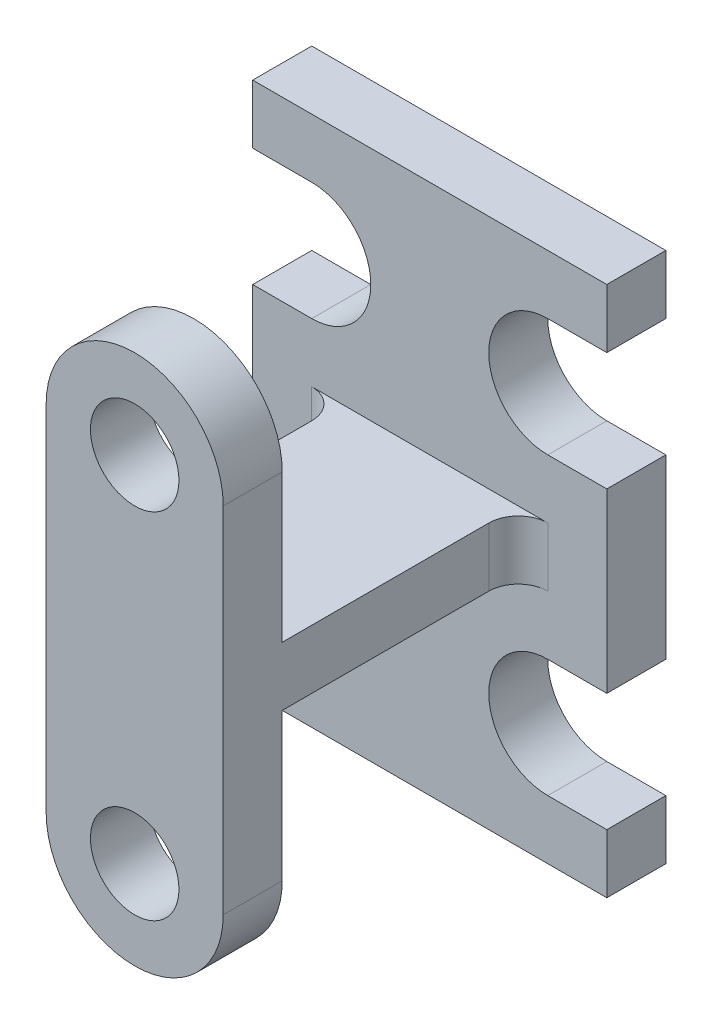
ISO-10303-21;
HEADER;
FILE_DESCRIPTION(('STEP AP214'),'2;1');
FILE_NAME('part.step','',(''),(''),'','','');
FILE_SCHEMA(('AUTOMOTIVE_DESIGN { 1 0 10303 214 1 1 1 1 }'));
ENDSEC;
DATA;
#1=APPLICATION_CONTEXT('core data for automotive mechanical design processes');
#2=APPLICATION_PROTOCOL_DEFINITION('international standard','automotive_design',2000,#1);
#3=PRODUCT_CONTEXT('',#1,'mechanical');
#4=PRODUCT('Part','Part','',(#3));
#5=PRODUCT_RELATED_PRODUCT_CATEGORY('part','',(#4));
#6=PRODUCT_DEFINITION_FORMATION('','',#4);
#7=PRODUCT_DEFINITION_CONTEXT('part definition',#1,'design');
#8=PRODUCT_DEFINITION('design','',#6,#7);
#9=PRODUCT_DEFINITION_SHAPE('','',#8);
#10=(LENGTH_UNIT() NAMED_UNIT(*) SI_UNIT(.MILLI.,.METRE.));
#11=(NAMED_UNIT(*) PLANE_ANGLE_UNIT() SI_UNIT($,.RADIAN.));
#12=(NAMED_UNIT(*) SI_UNIT($,.STERADIAN.) SOLID_ANGLE_UNIT());
#13=UNCERTAINTY_MEASURE_WITH_UNIT(LENGTH_MEASURE(1.E-05),#10,'distance_accuracy_value','');
#14=(GEOMETRIC_REPRESENTATION_CONTEXT(3) GLOBAL_UNCERTAINTY_ASSIGNED_CONTEXT((#13)) GLOBAL_UNIT_ASSIGNED_CONTEXT((#10,
#11,#12)) REPRESENTATION_CONTEXT('',''));
#15=CARTESIAN_POINT('',(0.,0.,0.));
#16=DIRECTION('',(0.,0.,1.));
#17=DIRECTION('',(1.,0.,0.));
#18=AXIS2_PLACEMENT_3D('',#15,#16,#17);
#19=CARTESIAN_POINT('',(3.,-3.5,1.));
#20=DIRECTION('',(-1.,0.,0.));
#21=DIRECTION('',(0.,-1.,0.));
#22=AXIS2_PLACEMENT_3D('',#19,#20,#21);
#23=PLANE('',#22);
#24=DIRECTION('',(0.,1.,0.));
#25=VECTOR('',#24,1.);
#26=CARTESIAN_POINT('',(3.,-3.5,0.));
#27=LINE('',#26,#25);
#28=CARTESIAN_POINT('',(3.,-4.5,0.));
#29=VERTEX_POINT('',#28);
#30=CARTESIAN_POINT('',(3.,-3.5,0.));
#31=VERTEX_POINT('',#30);
#32=EDGE_CURVE('E290',#29,#31,#27,.T.);
#33=ORIENTED_EDGE('',*,*,#32,.T.);
#34=DIRECTION('',(0.,0.,-1.));
#35=VECTOR('',#34,1.);
#36=CARTESIAN_POINT('',(3.,-3.5,1.));
#37=LINE('',#36,#35);
#38=CARTESIAN_POINT('',(3.,-3.5,1.));
#39=VERTEX_POINT('',#38);
#40=EDGE_CURVE('E426',#39,#31,#37,.T.);
#41=ORIENTED_EDGE('',*,*,#40,.F.);
#42=DIRECTION('',(0.,1.,0.));
#43=VECTOR('',#42,1.);
#44=CARTESIAN_POINT('',(3.,-3.5,1.));
#45=LINE('',#44,#43);
#46=CARTESIAN_POINT('',(3.,-4.5,1.));
#47=VERTEX_POINT('',#46);
#48=EDGE_CURVE('E288',#47,#39,#45,.T.);
#49=ORIENTED_EDGE('',*,*,#48,.F.);
#50=DIRECTION('',(0.,0.,-1.));
#51=VECTOR('',#50,1.);
#52=CARTESIAN_POINT('',(3.,-4.5,1.));
#53=LINE('',#52,#51);
#54=EDGE_CURVE('E329',#47,#29,#53,.T.);
#55=ORIENTED_EDGE('',*,*,#54,.T.);
#56=EDGE_LOOP('',(#33,#41,#49,#55));
#57=FACE_BOUND('',#56,.T.);
#58=ADVANCED_FACE('F39',(#57),#23,.F.);
#59=CARTESIAN_POINT('',(2.,-3.5,1.));
#60=DIRECTION('',(0.,-1.,0.));
#61=DIRECTION('',(0.,0.,-1.));
#62=AXIS2_PLACEMENT_3D('',#59,#60,#61);
#63=PLANE('',#62);
#64=DIRECTION('',(-1.,0.,0.));
#65=VECTOR('',#64,1.);
#66=CARTESIAN_POINT('',(2.,-3.5,0.));
#67=LINE('',#66,#65);
#68=CARTESIAN_POINT('',(2.,-3.5,0.));
#69=VERTEX_POINT('',#68);
#70=EDGE_CURVE('E334',#31,#69,#67,.T.);
#71=ORIENTED_EDGE('',*,*,#70,.T.);
#72=DIRECTION('',(0.,0.,-1.));
#73=VECTOR('',#72,1.);
#74=CARTESIAN_POINT('',(2.,-3.5,1.));
#75=LINE('',#74,#73);
#76=CARTESIAN_POINT('',(2.,-3.5,1.));
#77=VERTEX_POINT('',#76);
#78=EDGE_CURVE('E421',#77,#69,#75,.T.);
#79=ORIENTED_EDGE('',*,*,#78,.F.);
#80=DIRECTION('',(-1.,0.,0.));
#81=VECTOR('',#80,1.);
#82=CARTESIAN_POINT('',(2.,-3.5,1.));
#83=LINE('',#82,#81);
#84=EDGE_CURVE('E292',#39,#77,#83,.T.);
#85=ORIENTED_EDGE('',*,*,#84,.F.);
#86=ORIENTED_EDGE('',*,*,#40,.T.);
#87=EDGE_LOOP('',(#71,#79,#85,#86));
#88=FACE_BOUND('',#87,.T.);
#89=ADVANCED_FACE('F499',(#88),#63,.F.);
#90=CARTESIAN_POINT('',(2.,-2.5,1.));
#91=DIRECTION('',(0.,0.,-1.));
#92=DIRECTION('',(-1.,0.,0.));
#93=AXIS2_PLACEMENT_3D('',#90,#91,#92);
#94=CYLINDRICAL_SURFACE('',#93,0.999999999999999);
#95=CARTESIAN_POINT('',(2.,-2.5,0.));
#96=DIRECTION('',(0.,0.,-1.));
#97=DIRECTION('',(1.,0.,0.));
#98=AXIS2_PLACEMENT_3D('',#95,#96,#97);
#99=CIRCLE('',#98,0.999999999999999);
#100=CARTESIAN_POINT('',(2.,-1.5,0.));
#101=VERTEX_POINT('',#100);
#102=EDGE_CURVE('E333',#69,#101,#99,.T.);
#103=ORIENTED_EDGE('',*,*,#102,.T.);
#104=DIRECTION('',(0.,0.,-1.));
#105=VECTOR('',#104,1.);
#106=CARTESIAN_POINT('',(2.,-1.5,1.));
#107=LINE('',#106,#105);
#108=CARTESIAN_POINT('',(2.,-1.5,1.));
#109=VERTEX_POINT('',#108);
#110=EDGE_CURVE('E419',#109,#101,#107,.T.);
#111=ORIENTED_EDGE('',*,*,#110,.F.);
#112=CARTESIAN_POINT('',(2.,-2.5,1.));
#113=DIRECTION('',(0.,0.,-1.));
#114=DIRECTION('',(1.,0.,0.));
#115=AXIS2_PLACEMENT_3D('',#112,#113,#114);
#116=CIRCLE('',#115,0.999999999999999);
#117=EDGE_CURVE('E294',#77,#109,#116,.T.);
#118=ORIENTED_EDGE('',*,*,#117,.F.);
#119=ORIENTED_EDGE('',*,*,#78,.T.);
#120=EDGE_LOOP('',(#103,#111,#118,#119));
#121=FACE_BOUND('',#120,.T.);
#122=ADVANCED_FACE('F504',(#121),#94,.F.);
#123=CARTESIAN_POINT('',(2.,-1.5,1.));
#124=DIRECTION('',(0.,1.,0.));
#125=DIRECTION('',(-1.,0.,0.));
#126=AXIS2_PLACEMENT_3D('',#123,#124,#125);
#127=PLANE('',#126);
#128=DIRECTION('',(1.,0.,0.));
#129=VECTOR('',#128,1.);
#130=CARTESIAN_POINT('',(2.,-1.5,0.));
#131=LINE('',#130,#129);
#132=CARTESIAN_POINT('',(3.,-1.5,0.));
#133=VERTEX_POINT('',#132);
#134=EDGE_CURVE('E340',#101,#133,#131,.T.);
#135=ORIENTED_EDGE('',*,*,#134,.T.);
#136=DIRECTION('',(0.,0.,-1.));
#137=VECTOR('',#136,1.);
#138=CARTESIAN_POINT('',(3.,-1.5,1.));
#139=LINE('',#138,#137);
#140=CARTESIAN_POINT('',(3.,-1.5,1.));
#141=VERTEX_POINT('',#140);
#142=EDGE_CURVE('E417',#141,#133,#139,.T.);
#143=ORIENTED_EDGE('',*,*,#142,.F.);
#144=DIRECTION('',(1.,0.,0.));
#145=VECTOR('',#144,1.);
#146=CARTESIAN_POINT('',(2.,-1.5,1.));
#147=LINE('',#146,#145);
#148=EDGE_CURVE('E298',#109,#141,#147,.T.);
#149=ORIENTED_EDGE('',*,*,#148,.F.);
#150=ORIENTED_EDGE('',*,*,#110,.T.);
#151=EDGE_LOOP('',(#135,#143,#149,#150));
#152=FACE_BOUND('',#151,.T.);
#153=ADVANCED_FACE('F624',(#152),#127,.F.);
#154=CARTESIAN_POINT('',(3.,1.5,1.));
#155=DIRECTION('',(-1.,0.,0.));
#156=DIRECTION('',(0.,-1.,0.));
#157=AXIS2_PLACEMENT_3D('',#154,#155,#156);
#158=PLANE('',#157);
#159=DIRECTION('',(0.,1.,0.));
#160=VECTOR('',#159,1.);
#161=CARTESIAN_POINT('',(3.,1.5,0.));
#162=LINE('',#161,#160);
#163=CARTESIAN_POINT('',(3.,1.5,0.));
#164=VERTEX_POINT('',#163);
#165=EDGE_CURVE('E339',#133,#164,#162,.T.);
#166=ORIENTED_EDGE('',*,*,#165,.T.);
#167=DIRECTION('',(0.,0.,-1.));
#168=VECTOR('',#167,1.);
#169=CARTESIAN_POINT('',(3.,1.5,1.));
#170=LINE('',#169,#168);
#171=CARTESIAN_POINT('',(3.,1.5,1.));
#172=VERTEX_POINT('',#171);
#173=EDGE_CURVE('E414',#172,#164,#170,.T.);
#174=ORIENTED_EDGE('',*,*,#173,.F.);
#175=DIRECTION('',(0.,1.,0.));
#176=VECTOR('',#175,1.);
#177=CARTESIAN_POINT('',(3.,1.5,1.));
#178=LINE('',#177,#176);
#179=EDGE_CURVE('E296',#141,#172,#178,.T.);
#180=ORIENTED_EDGE('',*,*,#179,.F.);
#181=ORIENTED_EDGE('',*,*,#142,.T.);
#182=EDGE_LOOP('',(#166,#174,#180,#181));
#183=FACE_BOUND('',#182,.T.);
#184=ADVANCED_FACE('F616',(#183),#158,.F.);
#185=CARTESIAN_POINT('',(2.,1.5,1.));
#186=DIRECTION('',(0.,-1.,0.));
#187=DIRECTION('',(0.,0.,-1.));
#188=AXIS2_PLACEMENT_3D('',#185,#186,#187);
#189=PLANE('',#188);
#190=DIRECTION('',(-1.,0.,0.));
#191=VECTOR('',#190,1.);
#192=CARTESIAN_POINT('',(2.,1.5,0.));
#193=LINE('',#192,#191);
#194=CARTESIAN_POINT('',(2.,1.5,0.));
#195=VERTEX_POINT('',#194);
#196=EDGE_CURVE('E342',#164,#195,#193,.T.);
#197=ORIENTED_EDGE('',*,*,#196,.T.);
#198=DIRECTION('',(0.,0.,-1.));
#199=VECTOR('',#198,1.);
#200=CARTESIAN_POINT('',(2.,1.5,1.));
#201=LINE('',#200,#199);
#202=CARTESIAN_POINT('',(2.,1.5,1.));
#203=VERTEX_POINT('',#202);
#204=EDGE_CURVE('E412',#203,#195,#201,.T.);
#205=ORIENTED_EDGE('',*,*,#204,.F.);
#206=DIRECTION('',(-1.,0.,0.));
#207=VECTOR('',#206,1.);
#208=CARTESIAN_POINT('',(2.,1.5,1.));
#209=LINE('',#208,#207);
#210=EDGE_CURVE('E297',#172,#203,#209,.T.);
#211=ORIENTED_EDGE('',*,*,#210,.F.);
#212=ORIENTED_EDGE('',*,*,#173,.T.);
#213=EDGE_LOOP('',(#197,#205,#211,#212));
#214=FACE_BOUND('',#213,.T.);
#215=ADVANCED_FACE('F617',(#214),#189,.F.);
#216=CARTESIAN_POINT('',(2.,2.5,1.));
#217=DIRECTION('',(0.,0.,-1.));
#218=DIRECTION('',(-1.,0.,0.));
#219=AXIS2_PLACEMENT_3D('',#216,#217,#218);
#220=CYLINDRICAL_SURFACE('',#219,0.999999999999999);
#221=CARTESIAN_POINT('',(2.,2.5,0.));
#222=DIRECTION('',(0.,0.,-1.));
#223=DIRECTION('',(1.,0.,0.));
#224=AXIS2_PLACEMENT_3D('',#221,#222,#223);
#225=CIRCLE('',#224,0.999999999999999);
#226=CARTESIAN_POINT('',(2.,3.5,0.));
#227=VERTEX_POINT('',#226);
#228=EDGE_CURVE('E343',#195,#227,#225,.T.);
#229=ORIENTED_EDGE('',*,*,#228,.T.);
#230=DIRECTION('',(0.,0.,-1.));
#231=VECTOR('',#230,1.);
#232=CARTESIAN_POINT('',(2.,3.5,1.));
#233=LINE('',#232,#231);
#234=CARTESIAN_POINT('',(2.,3.5,1.));
#235=VERTEX_POINT('',#234);
#236=EDGE_CURVE('E406',#235,#227,#233,.T.);
#237=ORIENTED_EDGE('',*,*,#236,.F.);
#238=CARTESIAN_POINT('',(2.,2.5,1.));
#239=DIRECTION('',(0.,0.,-1.));
#240=DIRECTION('',(1.,0.,0.));
#241=AXIS2_PLACEMENT_3D('',#238,#239,#240);
#242=CIRCLE('',#241,0.999999999999999);
#243=EDGE_CURVE('E305',#203,#235,#242,.T.);
#244=ORIENTED_EDGE('',*,*,#243,.F.);
#245=ORIENTED_EDGE('',*,*,#204,.T.);
#246=EDGE_LOOP('',(#229,#237,#244,#245));
#247=FACE_BOUND('',#246,.T.);
#248=ADVANCED_FACE('F615',(#247),#220,.F.);
#249=CARTESIAN_POINT('',(2.,3.5,1.));
#250=DIRECTION('',(0.,1.,0.));
#251=DIRECTION('',(0.,0.,1.));
#252=AXIS2_PLACEMENT_3D('',#249,#250,#251);
#253=PLANE('',#252);
#254=DIRECTION('',(1.,0.,0.));
#255=VECTOR('',#254,1.);
#256=CARTESIAN_POINT('',(2.,3.5,0.));
#257=LINE('',#256,#255);
#258=CARTESIAN_POINT('',(3.,3.5,0.));
#259=VERTEX_POINT('',#258);
#260=EDGE_CURVE('E341',#227,#259,#257,.T.);
#261=ORIENTED_EDGE('',*,*,#260,.T.);
#262=DIRECTION('',(0.,0.,-1.));
#263=VECTOR('',#262,1.);
#264=CARTESIAN_POINT('',(3.,3.5,1.));
#265=LINE('',#264,#263);
#266=CARTESIAN_POINT('',(3.,3.5,1.));
#267=VERTEX_POINT('',#266);
#268=EDGE_CURVE('E403',#267,#259,#265,.T.);
#269=ORIENTED_EDGE('',*,*,#268,.F.);
#270=DIRECTION('',(1.,0.,0.));
#271=VECTOR('',#270,1.);
#272=CARTESIAN_POINT('',(2.,3.5,1.));
#273=LINE('',#272,#271);
#274=EDGE_CURVE('E304',#235,#267,#273,.T.);
#275=ORIENTED_EDGE('',*,*,#274,.F.);
#276=ORIENTED_EDGE('',*,*,#236,.T.);
#277=EDGE_LOOP('',(#261,#269,#275,#276));
#278=FACE_BOUND('',#277,.T.);
#279=ADVANCED_FACE('F609',(#278),#253,.F.);
#280=CARTESIAN_POINT('',(3.,4.5,1.));
#281=DIRECTION('',(-1.,0.,0.));
#282=DIRECTION('',(0.,-1.,0.));
#283=AXIS2_PLACEMENT_3D('',#280,#281,#282);
#284=PLANE('',#283);
#285=DIRECTION('',(0.,1.,0.));
#286=VECTOR('',#285,1.);
#287=CARTESIAN_POINT('',(3.,4.5,0.));
#288=LINE('',#287,#286);
#289=CARTESIAN_POINT('',(3.,4.5,0.));
#290=VERTEX_POINT('',#289);
#291=EDGE_CURVE('E350',#259,#290,#288,.T.);
#292=ORIENTED_EDGE('',*,*,#291,.T.);
#293=DIRECTION('',(0.,0.,-1.));
#294=VECTOR('',#293,1.);
#295=CARTESIAN_POINT('',(3.,4.5,1.));
#296=LINE('',#295,#294);
#297=CARTESIAN_POINT('',(3.,4.5,1.));
#298=VERTEX_POINT('',#297);
#299=EDGE_CURVE('E405',#298,#290,#296,.T.);
#300=ORIENTED_EDGE('',*,*,#299,.F.);
#301=DIRECTION('',(0.,1.,0.));
#302=VECTOR('',#301,1.);
#303=CARTESIAN_POINT('',(3.,4.5,1.));
#304=LINE('',#303,#302);
#305=EDGE_CURVE('E308',#267,#298,#304,.T.);
#306=ORIENTED_EDGE('',*,*,#305,.F.);
#307=ORIENTED_EDGE('',*,*,#268,.T.);
#308=EDGE_LOOP('',(#292,#300,#306,#307));
#309=FACE_BOUND('',#308,.T.);
#310=ADVANCED_FACE('F603',(#309),#284,.F.);
#311=CARTESIAN_POINT('',(-3.,4.5,1.));
#312=DIRECTION('',(0.,-1.,0.));
#313=DIRECTION('',(0.,0.,-1.));
#314=AXIS2_PLACEMENT_3D('',#311,#312,#313);
#315=PLANE('',#314);
#316=DIRECTION('',(-1.,0.,0.));
#317=VECTOR('',#316,1.);
#318=CARTESIAN_POINT('',(-3.,4.5,0.));
#319=LINE('',#318,#317);
#320=CARTESIAN_POINT('',(-3.,4.5,0.));
#321=VERTEX_POINT('',#320);
#322=EDGE_CURVE('E349',#290,#321,#319,.T.);
#323=ORIENTED_EDGE('',*,*,#322,.T.);
#324=DIRECTION('',(0.,0.,-1.));
#325=VECTOR('',#324,1.);
#326=CARTESIAN_POINT('',(-3.,4.5,1.));
#327=LINE('',#326,#325);
#328=CARTESIAN_POINT('',(-3.,4.5,1.));
#329=VERTEX_POINT('',#328);
#330=EDGE_CURVE('E399',#329,#321,#327,.T.);
#331=ORIENTED_EDGE('',*,*,#330,.F.);
#332=DIRECTION('',(-1.,0.,0.));
#333=VECTOR('',#332,1.);
#334=CARTESIAN_POINT('',(-3.,4.5,1.));
#335=LINE('',#334,#333);
#336=EDGE_CURVE('E306',#298,#329,#335,.T.);
#337=ORIENTED_EDGE('',*,*,#336,.F.);
#338=ORIENTED_EDGE('',*,*,#299,.T.);
#339=EDGE_LOOP('',(#323,#331,#337,#338));
#340=FACE_BOUND('',#339,.T.);
#341=ADVANCED_FACE('F599',(#340),#315,.F.);
#342=CARTESIAN_POINT('',(-3.,4.5,1.));
#343=DIRECTION('',(1.,0.,0.));
#344=DIRECTION('',(0.,0.,-1.));
#345=AXIS2_PLACEMENT_3D('',#342,#343,#344);
#346=PLANE('',#345);
#347=DIRECTION('',(0.,-1.,0.));
#348=VECTOR('',#347,1.);
#349=CARTESIAN_POINT('',(-3.,4.5,0.));
#350=LINE('',#349,#348);
#351=CARTESIAN_POINT('',(-3.,3.5,0.));
#352=VERTEX_POINT('',#351);
#353=EDGE_CURVE('E353',#321,#352,#350,.T.);
#354=ORIENTED_EDGE('',*,*,#353,.T.);
#355=DIRECTION('',(0.,0.,-1.));
#356=VECTOR('',#355,1.);
#357=CARTESIAN_POINT('',(-3.,3.5,1.));
#358=LINE('',#357,#356);
#359=CARTESIAN_POINT('',(-3.,3.5,1.));
#360=VERTEX_POINT('',#359);
#361=EDGE_CURVE('E397',#360,#352,#358,.T.);
#362=ORIENTED_EDGE('',*,*,#361,.F.);
#363=DIRECTION('',(0.,-1.,0.));
#364=VECTOR('',#363,1.);
#365=CARTESIAN_POINT('',(-3.,4.5,1.));
#366=LINE('',#365,#364);
#367=EDGE_CURVE('E309',#329,#360,#366,.T.);
#368=ORIENTED_EDGE('',*,*,#367,.F.);
#369=ORIENTED_EDGE('',*,*,#330,.T.);
#370=EDGE_LOOP('',(#354,#362,#368,#369));
#371=FACE_BOUND('',#370,.T.);
#372=ADVANCED_FACE('F596',(#371),#346,.F.);
#373=CARTESIAN_POINT('',(-3.,3.5,1.));
#374=DIRECTION('',(0.,1.,0.));
#375=DIRECTION('',(0.,0.,1.));
#376=AXIS2_PLACEMENT_3D('',#373,#374,#375);
#377=PLANE('',#376);
#378=DIRECTION('',(1.,0.,0.));
#379=VECTOR('',#378,1.);
#380=CARTESIAN_POINT('',(-3.,3.5,0.));
#381=LINE('',#380,#379);
#382=CARTESIAN_POINT('',(-2.,3.5,0.));
#383=VERTEX_POINT('',#382);
#384=EDGE_CURVE('E351',#352,#383,#381,.T.);
#385=ORIENTED_EDGE('',*,*,#384,.T.);
#386=DIRECTION('',(0.,0.,-1.));
#387=VECTOR('',#386,1.);
#388=CARTESIAN_POINT('',(-2.,3.5,1.));
#389=LINE('',#388,#387);
#390=CARTESIAN_POINT('',(-2.,3.5,1.));
#391=VERTEX_POINT('',#390);
#392=EDGE_CURVE('E391',#391,#383,#389,.T.);
#393=ORIENTED_EDGE('',*,*,#392,.F.);
#394=DIRECTION('',(1.,0.,0.));
#395=VECTOR('',#394,1.);
#396=CARTESIAN_POINT('',(-3.,3.5,1.));
#397=LINE('',#396,#395);
#398=EDGE_CURVE('E315',#360,#391,#397,.T.);
#399=ORIENTED_EDGE('',*,*,#398,.F.);
#400=ORIENTED_EDGE('',*,*,#361,.T.);
#401=EDGE_LOOP('',(#385,#393,#399,#400));
#402=FACE_BOUND('',#401,.T.);
#403=ADVANCED_FACE('F595',(#402),#377,.F.);
#404=CARTESIAN_POINT('',(-2.,2.5,1.));
#405=DIRECTION('',(0.,0.,-1.));
#406=DIRECTION('',(-1.,0.,0.));
#407=AXIS2_PLACEMENT_3D('',#404,#405,#406);
#408=CYLINDRICAL_SURFACE('',#407,0.999999999999999);
#409=CARTESIAN_POINT('',(-2.,2.5,0.));
#410=DIRECTION('',(0.,0.,-1.));
#411=DIRECTION('',(1.,0.,0.));
#412=AXIS2_PLACEMENT_3D('',#409,#410,#411);
#413=CIRCLE('',#412,0.999999999999999);
#414=CARTESIAN_POINT('',(-2.,1.5,0.));
#415=VERTEX_POINT('',#414);
#416=EDGE_CURVE('E352',#383,#415,#413,.T.);
#417=ORIENTED_EDGE('',*,*,#416,.T.);
#418=DIRECTION('',(0.,0.,-1.));
#419=VECTOR('',#418,1.);
#420=CARTESIAN_POINT('',(-2.,1.5,1.));
#421=LINE('',#420,#419);
#422=CARTESIAN_POINT('',(-2.,1.5,1.));
#423=VERTEX_POINT('',#422);
#424=EDGE_CURVE('E388',#423,#415,#421,.T.);
#425=ORIENTED_EDGE('',*,*,#424,.F.);
#426=CARTESIAN_POINT('',(-2.,2.5,1.));
#427=DIRECTION('',(0.,0.,-1.));
#428=DIRECTION('',(1.,0.,0.));
#429=AXIS2_PLACEMENT_3D('',#426,#427,#428);
#430=CIRCLE('',#429,0.999999999999999);
#431=EDGE_CURVE('E314',#391,#423,#430,.T.);
#432=ORIENTED_EDGE('',*,*,#431,.F.);
#433=ORIENTED_EDGE('',*,*,#392,.T.);
#434=EDGE_LOOP('',(#417,#425,#432,#433));
#435=FACE_BOUND('',#434,.T.);
#436=ADVANCED_FACE('F586',(#435),#408,.F.);
#437=CARTESIAN_POINT('',(-3.,1.5,1.));
#438=DIRECTION('',(0.,-1.,0.));
#439=DIRECTION('',(0.,0.,-1.));
#440=AXIS2_PLACEMENT_3D('',#437,#438,#439);
#441=PLANE('',#440);
#442=DIRECTION('',(-1.,0.,0.));
#443=VECTOR('',#442,1.);
#444=CARTESIAN_POINT('',(-3.,1.5,0.));
#445=LINE('',#444,#443);
#446=CARTESIAN_POINT('',(-3.,1.5,0.));
#447=VERTEX_POINT('',#446);
#448=EDGE_CURVE('E360',#415,#447,#445,.T.);
#449=ORIENTED_EDGE('',*,*,#448,.T.);
#450=DIRECTION('',(0.,0.,-1.));
#451=VECTOR('',#450,1.);
#452=CARTESIAN_POINT('',(-3.,1.5,1.));
#453=LINE('',#452,#451);
#454=CARTESIAN_POINT('',(-3.,1.5,1.));
#455=VERTEX_POINT('',#454);
#456=EDGE_CURVE('E390',#455,#447,#453,.T.);
#457=ORIENTED_EDGE('',*,*,#456,.F.);
#458=DIRECTION('',(-1.,0.,0.));
#459=VECTOR('',#458,1.);
#460=CARTESIAN_POINT('',(-3.,1.5,1.));
#461=LINE('',#460,#459);
#462=EDGE_CURVE('E316',#423,#455,#461,.T.);
#463=ORIENTED_EDGE('',*,*,#462,.F.);
#464=ORIENTED_EDGE('',*,*,#424,.T.);
#465=EDGE_LOOP('',(#449,#457,#463,#464));
#466=FACE_BOUND('',#465,.T.);
#467=ADVANCED_FACE('F585',(#466),#441,.F.);
#468=CARTESIAN_POINT('',(-3.,1.5,1.));
#469=DIRECTION('',(1.,0.,0.));
#470=DIRECTION('',(0.,1.,0.));
#471=AXIS2_PLACEMENT_3D('',#468,#469,#470);
#472=PLANE('',#471);
#473=DIRECTION('',(0.,-1.,0.));
#474=VECTOR('',#473,1.);
#475=CARTESIAN_POINT('',(-3.,1.5,0.));
#476=LINE('',#475,#474);
#477=CARTESIAN_POINT('',(-3.,-1.5,0.));
#478=VERTEX_POINT('',#477);
#479=EDGE_CURVE('E359',#447,#478,#476,.T.);
#480=ORIENTED_EDGE('',*,*,#479,.T.);
#481=DIRECTION('',(0.,0.,-1.));
#482=VECTOR('',#481,1.);
#483=CARTESIAN_POINT('',(-3.,-1.5,1.));
#484=LINE('',#483,#482);
#485=CARTESIAN_POINT('',(-3.,-1.5,1.));
#486=VERTEX_POINT('',#485);
#487=EDGE_CURVE('E383',#486,#478,#484,.T.);
#488=ORIENTED_EDGE('',*,*,#487,.F.);
#489=DIRECTION('',(0.,-1.,0.));
#490=VECTOR('',#489,1.);
#491=CARTESIAN_POINT('',(-3.,1.5,1.));
#492=LINE('',#491,#490);
#493=EDGE_CURVE('E318',#455,#486,#492,.T.);
#494=ORIENTED_EDGE('',*,*,#493,.F.);
#495=ORIENTED_EDGE('',*,*,#456,.T.);
#496=EDGE_LOOP('',(#480,#488,#494,#495));
#497=FACE_BOUND('',#496,.T.);
#498=ADVANCED_FACE('F576',(#497),#472,.F.);
#499=CARTESIAN_POINT('',(-3.,-1.5,1.));
#500=DIRECTION('',(0.,1.,0.));
#501=DIRECTION('',(0.,0.,1.));
#502=AXIS2_PLACEMENT_3D('',#499,#500,#501);
#503=PLANE('',#502);
#504=DIRECTION('',(1.,0.,0.));
#505=VECTOR('',#504,1.);
#506=CARTESIAN_POINT('',(-3.,-1.5,0.));
#507=LINE('',#506,#505);
#508=CARTESIAN_POINT('',(-2.,-1.5,0.));
#509=VERTEX_POINT('',#508);
#510=EDGE_CURVE('E363',#478,#509,#507,.T.);
#511=ORIENTED_EDGE('',*,*,#510,.T.);
#512=DIRECTION('',(0.,0.,-1.));
#513=VECTOR('',#512,1.);
#514=CARTESIAN_POINT('',(-2.,-1.5,1.));
#515=LINE('',#514,#513);
#516=CARTESIAN_POINT('',(-2.,-1.5,1.));
#517=VERTEX_POINT('',#516);
#518=EDGE_CURVE('E381',#517,#509,#515,.T.);
#519=ORIENTED_EDGE('',*,*,#518,.F.);
#520=DIRECTION('',(1.,0.,0.));
#521=VECTOR('',#520,1.);
#522=CARTESIAN_POINT('',(-3.,-1.5,1.));
#523=LINE('',#522,#521);
#524=EDGE_CURVE('E319',#486,#517,#523,.T.);
#525=ORIENTED_EDGE('',*,*,#524,.F.);
#526=ORIENTED_EDGE('',*,*,#487,.T.);
#527=EDGE_LOOP('',(#511,#519,#525,#526));
#528=FACE_BOUND('',#527,.T.);
#529=ADVANCED_FACE('F577',(#528),#503,.F.);
#530=CARTESIAN_POINT('',(-2.,-2.5,1.));
#531=DIRECTION('',(0.,0.,-1.));
#532=DIRECTION('',(-1.,0.,0.));
#533=AXIS2_PLACEMENT_3D('',#530,#531,#532);
#534=CYLINDRICAL_SURFACE('',#533,0.999999999999999);
#535=CARTESIAN_POINT('',(-2.,-2.5,0.));
#536=DIRECTION('',(0.,0.,-1.));
#537=DIRECTION('',(1.,0.,0.));
#538=AXIS2_PLACEMENT_3D('',#535,#536,#537);
#539=CIRCLE('',#538,0.999999999999999);
#540=CARTESIAN_POINT('',(-2.,-3.5,0.));
#541=VERTEX_POINT('',#540);
#542=EDGE_CURVE('E361',#509,#541,#539,.T.);
#543=ORIENTED_EDGE('',*,*,#542,.T.);
#544=DIRECTION('',(0.,0.,-1.));
#545=VECTOR('',#544,1.);
#546=CARTESIAN_POINT('',(-2.,-3.5,1.));
#547=LINE('',#546,#545);
#548=CARTESIAN_POINT('',(-2.,-3.5,1.));
#549=VERTEX_POINT('',#548);
#550=EDGE_CURVE('E378',#549,#541,#547,.T.);
#551=ORIENTED_EDGE('',*,*,#550,.F.);
#552=CARTESIAN_POINT('',(-2.,-2.5,1.));
#553=DIRECTION('',(0.,0.,-1.));
#554=DIRECTION('',(1.,0.,0.));
#555=AXIS2_PLACEMENT_3D('',#552,#553,#554);
#556=CIRCLE('',#555,0.999999999999999);
#557=EDGE_CURVE('E325',#517,#549,#556,.T.);
#558=ORIENTED_EDGE('',*,*,#557,.F.);
#559=ORIENTED_EDGE('',*,*,#518,.T.);
#560=EDGE_LOOP('',(#543,#551,#558,#559));
#561=FACE_BOUND('',#560,.T.);
#562=ADVANCED_FACE('F575',(#561),#534,.F.);
#563=CARTESIAN_POINT('',(-3.,-3.5,1.));
#564=DIRECTION('',(0.,-1.,0.));
#565=DIRECTION('',(0.,0.,-1.));
#566=AXIS2_PLACEMENT_3D('',#563,#564,#565);
#567=PLANE('',#566);
#568=DIRECTION('',(-1.,0.,0.));
#569=VECTOR('',#568,1.);
#570=CARTESIAN_POINT('',(-3.,-3.5,0.));
#571=LINE('',#570,#569);
#572=CARTESIAN_POINT('',(-3.,-3.5,0.));
#573=VERTEX_POINT('',#572);
#574=EDGE_CURVE('E364',#541,#573,#571,.T.);
#575=ORIENTED_EDGE('',*,*,#574,.T.);
#576=DIRECTION('',(0.,0.,-1.));
#577=VECTOR('',#576,1.);
#578=CARTESIAN_POINT('',(-3.,-3.5,1.));
#579=LINE('',#578,#577);
#580=CARTESIAN_POINT('',(-3.,-3.5,1.));
#581=VERTEX_POINT('',#580);
#582=EDGE_CURVE('E374',#581,#573,#579,.T.);
#583=ORIENTED_EDGE('',*,*,#582,.F.);
#584=DIRECTION('',(-1.,0.,0.));
#585=VECTOR('',#584,1.);
#586=CARTESIAN_POINT('',(-3.,-3.5,1.));
#587=LINE('',#586,#585);
#588=EDGE_CURVE('E322',#549,#581,#587,.T.);
#589=ORIENTED_EDGE('',*,*,#588,.F.);
#590=ORIENTED_EDGE('',*,*,#550,.T.);
#591=EDGE_LOOP('',(#575,#583,#589,#590));
#592=FACE_BOUND('',#591,.T.);
#593=ADVANCED_FACE('F566',(#592),#567,.F.);
#594=CARTESIAN_POINT('',(-3.,-3.5,1.));
#595=DIRECTION('',(1.,0.,0.));
#596=DIRECTION('',(0.,1.,0.));
#597=AXIS2_PLACEMENT_3D('',#594,#595,#596);
#598=PLANE('',#597);
#599=DIRECTION('',(0.,-1.,0.));
#600=VECTOR('',#599,1.);
#601=CARTESIAN_POINT('',(-3.,-3.5,0.));
#602=LINE('',#601,#600);
#603=CARTESIAN_POINT('',(-3.,-4.5,0.));
#604=VERTEX_POINT('',#603);
#605=EDGE_CURVE('E370',#573,#604,#602,.T.);
#606=ORIENTED_EDGE('',*,*,#605,.T.);
#607=DIRECTION('',(0.,0.,-1.));
#608=VECTOR('',#607,1.);
#609=CARTESIAN_POINT('',(-3.,-4.5,1.));
#610=LINE('',#609,#608);
#611=CARTESIAN_POINT('',(-3.,-4.5,1.));
#612=VERTEX_POINT('',#611);
#613=EDGE_CURVE('E375',#612,#604,#610,.T.);
#614=ORIENTED_EDGE('',*,*,#613,.F.);
#615=DIRECTION('',(0.,-1.,0.));
#616=VECTOR('',#615,1.);
#617=CARTESIAN_POINT('',(-3.,-3.5,1.));
#618=LINE('',#617,#616);
#619=EDGE_CURVE('E326',#581,#612,#618,.T.);
#620=ORIENTED_EDGE('',*,*,#619,.F.);
#621=ORIENTED_EDGE('',*,*,#582,.T.);
#622=EDGE_LOOP('',(#606,#614,#620,#621));
#623=FACE_BOUND('',#622,.T.);
#624=ADVANCED_FACE('F564',(#623),#598,.F.);
#625=CARTESIAN_POINT('',(-3.,-4.5,1.));
#626=DIRECTION('',(0.,1.,0.));
#627=DIRECTION('',(0.,0.,1.));
#628=AXIS2_PLACEMENT_3D('',#625,#626,#627);
#629=PLANE('',#628);
#630=DIRECTION('',(1.,0.,0.));
#631=VECTOR('',#630,1.);
#632=CARTESIAN_POINT('',(-3.,-4.5,0.));
#633=LINE('',#632,#631);
#634=EDGE_CURVE('E295',#604,#29,#633,.T.);
#635=ORIENTED_EDGE('',*,*,#634,.T.);
#636=ORIENTED_EDGE('',*,*,#54,.F.);
#637=DIRECTION('',(1.,0.,0.));
#638=VECTOR('',#637,1.);
#639=CARTESIAN_POINT('',(-3.,-4.5,1.));
#640=LINE('',#639,#638);
#641=EDGE_CURVE('E327',#612,#47,#640,.T.);
#642=ORIENTED_EDGE('',*,*,#641,.F.);
#643=ORIENTED_EDGE('',*,*,#613,.T.);
#644=EDGE_LOOP('',(#635,#636,#642,#643));
#645=FACE_BOUND('',#644,.T.);
#646=ADVANCED_FACE('F559',(#645),#629,.F.);
#647=CARTESIAN_POINT('',(-2.,-2.5,1.));
#648=DIRECTION('',(0.,0.,1.));
#649=DIRECTION('',(1.,0.,0.));
#650=AXIS2_PLACEMENT_3D('',#647,#648,#649);
#651=PLANE('',#650);
#652=DIRECTION('',(1.,0.,0.));
#653=VECTOR('',#652,1.);
#654=CARTESIAN_POINT('',(1.5,-0.5,1.));
#655=LINE('',#654,#653);
#656=CARTESIAN_POINT('',(-2.,-0.5,1.));
#657=VERTEX_POINT('',#656);
#658=CARTESIAN_POINT('',(2.,-0.5,1.));
#659=VERTEX_POINT('',#658);
#660=EDGE_CURVE('E53',#657,#659,#655,.T.);
#661=ORIENTED_EDGE('',*,*,#660,.F.);
#662=DIRECTION('',(0.,-1.,0.));
#663=VECTOR('',#662,1.);
#664=CARTESIAN_POINT('',(-2.,-2.5,1.));
#665=LINE('',#664,#663);
#666=CARTESIAN_POINT('',(-2.,0.5,1.));
#667=VERTEX_POINT('',#666);
#668=EDGE_CURVE('E442',#657,#667,#665,.F.);
#669=ORIENTED_EDGE('',*,*,#668,.T.);
#670=DIRECTION('',(-1.,0.,0.));
#671=VECTOR('',#670,1.);
#672=CARTESIAN_POINT('',(1.5,0.5,1.));
#673=LINE('',#672,#671);
#674=CARTESIAN_POINT('',(2.,0.5,1.));
#675=VERTEX_POINT('',#674);
#676=EDGE_CURVE('E63',#675,#667,#673,.T.);
#677=ORIENTED_EDGE('',*,*,#676,.F.);
#678=DIRECTION('',(0.,1.,0.));
#679=VECTOR('',#678,1.);
#680=CARTESIAN_POINT('',(2.,-2.5,1.));
#681=LINE('',#680,#679);
#682=EDGE_CURVE('E435',#675,#659,#681,.F.);
#683=ORIENTED_EDGE('',*,*,#682,.T.);
#684=EDGE_LOOP('',(#661,#669,#677,#683));
#685=FACE_BOUND('',#684,.T.);
#686=ORIENTED_EDGE('',*,*,#48,.T.);
#687=ORIENTED_EDGE('',*,*,#84,.T.);
#688=ORIENTED_EDGE('',*,*,#117,.T.);
#689=ORIENTED_EDGE('',*,*,#148,.T.);
#690=ORIENTED_EDGE('',*,*,#179,.T.);
#691=ORIENTED_EDGE('',*,*,#210,.T.);
#692=ORIENTED_EDGE('',*,*,#243,.T.);
#693=ORIENTED_EDGE('',*,*,#274,.T.);
#694=ORIENTED_EDGE('',*,*,#305,.T.);
#695=ORIENTED_EDGE('',*,*,#336,.T.);
#696=ORIENTED_EDGE('',*,*,#367,.T.);
#697=ORIENTED_EDGE('',*,*,#398,.T.);
#698=ORIENTED_EDGE('',*,*,#431,.T.);
#699=ORIENTED_EDGE('',*,*,#462,.T.);
#700=ORIENTED_EDGE('',*,*,#493,.T.);
#701=ORIENTED_EDGE('',*,*,#524,.T.);
#702=ORIENTED_EDGE('',*,*,#557,.T.);
#703=ORIENTED_EDGE('',*,*,#588,.T.);
#704=ORIENTED_EDGE('',*,*,#619,.T.);
#705=ORIENTED_EDGE('',*,*,#641,.T.);
#706=EDGE_LOOP('',(#686,#687,#688,#689,#690,#691,#692,#693,#694,#695,#696,#697,#698,#699,#700,
#701,#702,#703,#704,#705));
#707=FACE_BOUND('',#706,.T.);
#708=ADVANCED_FACE('F449',(#685,#707),#651,.T.);
#709=CARTESIAN_POINT('',(-2.,-2.5,0.));
#710=DIRECTION('',(0.,0.,1.));
#711=DIRECTION('',(1.,0.,0.));
#712=AXIS2_PLACEMENT_3D('',#709,#710,#711);
#713=PLANE('',#712);
#714=ORIENTED_EDGE('',*,*,#32,.F.);
#715=ORIENTED_EDGE('',*,*,#634,.F.);
#716=ORIENTED_EDGE('',*,*,#605,.F.);
#717=ORIENTED_EDGE('',*,*,#574,.F.);
#718=ORIENTED_EDGE('',*,*,#542,.F.);
#719=ORIENTED_EDGE('',*,*,#510,.F.);
#720=ORIENTED_EDGE('',*,*,#479,.F.);
#721=ORIENTED_EDGE('',*,*,#448,.F.);
#722=ORIENTED_EDGE('',*,*,#416,.F.);
#723=ORIENTED_EDGE('',*,*,#384,.F.);
#724=ORIENTED_EDGE('',*,*,#353,.F.);
#725=ORIENTED_EDGE('',*,*,#322,.F.);
#726=ORIENTED_EDGE('',*,*,#291,.F.);
#727=ORIENTED_EDGE('',*,*,#260,.F.);
#728=ORIENTED_EDGE('',*,*,#228,.F.);
#729=ORIENTED_EDGE('',*,*,#196,.F.);
#730=ORIENTED_EDGE('',*,*,#165,.F.);
#731=ORIENTED_EDGE('',*,*,#134,.F.);
#732=ORIENTED_EDGE('',*,*,#102,.F.);
#733=ORIENTED_EDGE('',*,*,#70,.F.);
#734=EDGE_LOOP('',(#714,#715,#716,#717,#718,#719,#720,#721,#722,#723,#724,#725,#726,#727,#728,
#729,#730,#731,#732,#733));
#735=FACE_BOUND('',#734,.T.);
#736=ADVANCED_FACE('F560',(#735),#713,.F.);
#737=CARTESIAN_POINT('',(-1.5,-0.5,5.));
#738=DIRECTION('',(1.,0.,0.));
#739=DIRECTION('',(0.,0.,-1.));
#740=AXIS2_PLACEMENT_3D('',#737,#738,#739);
#741=PLANE('',#740);
#742=DIRECTION('',(0.,0.,-1.));
#743=VECTOR('',#742,1.);
#744=CARTESIAN_POINT('',(-1.5,0.5,5.));
#745=LINE('',#744,#743);
#746=CARTESIAN_POINT('',(-1.5,0.5,5.));
#747=VERTEX_POINT('',#746);
#748=CARTESIAN_POINT('',(-1.5,0.5,1.5));
#749=VERTEX_POINT('',#748);
#750=EDGE_CURVE('E273',#747,#749,#745,.T.);
#751=ORIENTED_EDGE('',*,*,#750,.T.);
#752=DIRECTION('',(0.,-1.,0.));
#753=VECTOR('',#752,1.);
#754=CARTESIAN_POINT('',(-1.5,-0.5,1.5));
#755=LINE('',#754,#753);
#756=CARTESIAN_POINT('',(-1.5,-0.5,1.5));
#757=VERTEX_POINT('',#756);
#758=EDGE_CURVE('E437',#749,#757,#755,.T.);
#759=ORIENTED_EDGE('',*,*,#758,.T.);
#760=DIRECTION('',(0.,0.,-1.));
#761=VECTOR('',#760,1.);
#762=CARTESIAN_POINT('',(-1.5,-0.5,5.));
#763=LINE('',#762,#761);
#764=CARTESIAN_POINT('',(-1.5,-0.5,5.));
#765=VERTEX_POINT('',#764);
#766=EDGE_CURVE('E284',#765,#757,#763,.T.);
#767=ORIENTED_EDGE('',*,*,#766,.F.);
#768=DIRECTION('',(0.,-1.,0.));
#769=VECTOR('',#768,1.);
#770=CARTESIAN_POINT('',(-1.5,3.,5.));
#771=LINE('',#770,#769);
#772=CARTESIAN_POINT('',(-1.5,-3.,5.));
#773=VERTEX_POINT('',#772);
#774=EDGE_CURVE('E478',#765,#773,#771,.T.);
#775=ORIENTED_EDGE('',*,*,#774,.T.);
#776=DIRECTION('',(0.,0.,-1.));
#777=VECTOR('',#776,1.);
#778=CARTESIAN_POINT('',(-1.5,-3.,6.));
#779=LINE('',#778,#777);
#780=CARTESIAN_POINT('',(-1.5,-3.,6.));
#781=VERTEX_POINT('',#780);
#782=EDGE_CURVE('E244',#781,#773,#779,.T.);
#783=ORIENTED_EDGE('',*,*,#782,.F.);
#784=DIRECTION('',(0.,-1.,0.));
#785=VECTOR('',#784,1.);
#786=CARTESIAN_POINT('',(-1.5,3.,6.));
#787=LINE('',#786,#785);
#788=CARTESIAN_POINT('',(-1.5,3.,6.));
#789=VERTEX_POINT('',#788);
#790=EDGE_CURVE('E231',#789,#781,#787,.T.);
#791=ORIENTED_EDGE('',*,*,#790,.F.);
#792=DIRECTION('',(0.,0.,-1.));
#793=VECTOR('',#792,1.);
#794=CARTESIAN_POINT('',(-1.5,3.,6.));
#795=LINE('',#794,#793);
#796=CARTESIAN_POINT('',(-1.5,3.,5.));
#797=VERTEX_POINT('',#796);
#798=EDGE_CURVE('E243',#789,#797,#795,.T.);
#799=ORIENTED_EDGE('',*,*,#798,.T.);
#800=EDGE_CURVE('E476',#797,#747,#771,.T.);
#801=ORIENTED_EDGE('',*,*,#800,.T.);
#802=EDGE_LOOP('',(#751,#759,#767,#775,#783,#791,#799,#801));
#803=FACE_BOUND('',#802,.T.);
#804=ADVANCED_FACE('F236',(#803),#741,.F.);
#805=CARTESIAN_POINT('',(1.5,-0.5,5.));
#806=DIRECTION('',(0.,1.,0.));
#807=DIRECTION('',(-1.,0.,0.));
#808=AXIS2_PLACEMENT_3D('',#805,#806,#807);
#809=PLANE('',#808);
#810=ORIENTED_EDGE('',*,*,#660,.T.);
#811=CARTESIAN_POINT('',(2.,-0.5,1.5));
#812=DIRECTION('',(0.,1.,0.));
#813=DIRECTION('',(-1.,0.,0.));
#814=AXIS2_PLACEMENT_3D('',#811,#812,#813);
#815=CIRCLE('',#814,0.5);
#816=CARTESIAN_POINT('',(1.5,-0.5,1.5));
#817=VERTEX_POINT('',#816);
#818=EDGE_CURVE('E436',#659,#817,#815,.T.);
#819=ORIENTED_EDGE('',*,*,#818,.T.);
#820=DIRECTION('',(0.,0.,-1.));
#821=VECTOR('',#820,1.);
#822=CARTESIAN_POINT('',(1.5,-0.5,5.));
#823=LINE('',#822,#821);
#824=CARTESIAN_POINT('',(1.5,-0.5,5.));
#825=VERTEX_POINT('',#824);
#826=EDGE_CURVE('E283',#825,#817,#823,.T.);
#827=ORIENTED_EDGE('',*,*,#826,.F.);
#828=DIRECTION('',(1.,0.,0.));
#829=VECTOR('',#828,1.);
#830=CARTESIAN_POINT('',(1.5,-0.5,5.));
#831=LINE('',#830,#829);
#832=EDGE_CURVE('E267',#765,#825,#831,.T.);
#833=ORIENTED_EDGE('',*,*,#832,.F.);
#834=ORIENTED_EDGE('',*,*,#766,.T.);
#835=CARTESIAN_POINT('',(-2.,-0.5,1.5));
#836=DIRECTION('',(0.,1.,0.));
#837=DIRECTION('',(-1.,0.,0.));
#838=AXIS2_PLACEMENT_3D('',#835,#836,#837);
#839=CIRCLE('',#838,0.5);
#840=EDGE_CURVE('E50',#757,#657,#839,.T.);
#841=ORIENTED_EDGE('',*,*,#840,.T.);
#842=EDGE_LOOP('',(#810,#819,#827,#833,#834,#841));
#843=FACE_BOUND('',#842,.T.);
#844=ADVANCED_FACE('F441',(#843),#809,.F.);
#845=CARTESIAN_POINT('',(1.5,-0.5,5.));
#846=DIRECTION('',(-1.,0.,0.));
#847=DIRECTION('',(0.,-1.,0.));
#848=AXIS2_PLACEMENT_3D('',#845,#846,#847);
#849=PLANE('',#848);
#850=ORIENTED_EDGE('',*,*,#826,.T.);
#851=DIRECTION('',(0.,1.,0.));
#852=VECTOR('',#851,1.);
#853=CARTESIAN_POINT('',(1.5,-0.5,1.5));
#854=LINE('',#853,#852);
#855=CARTESIAN_POINT('',(1.5,0.5,1.5));
#856=VERTEX_POINT('',#855);
#857=EDGE_CURVE('E427',#817,#856,#854,.T.);
#858=ORIENTED_EDGE('',*,*,#857,.T.);
#859=DIRECTION('',(0.,0.,-1.));
#860=VECTOR('',#859,1.);
#861=CARTESIAN_POINT('',(1.5,0.5,5.));
#862=LINE('',#861,#860);
#863=CARTESIAN_POINT('',(1.5,0.5,5.));
#864=VERTEX_POINT('',#863);
#865=EDGE_CURVE('E279',#864,#856,#862,.T.);
#866=ORIENTED_EDGE('',*,*,#865,.F.);
#867=DIRECTION('',(0.,1.,0.));
#868=VECTOR('',#867,1.);
#869=CARTESIAN_POINT('',(1.5,3.,5.));
#870=LINE('',#869,#868);
#871=CARTESIAN_POINT('',(1.5,3.,5.));
#872=VERTEX_POINT('',#871);
#873=EDGE_CURVE('E467',#864,#872,#870,.T.);
#874=ORIENTED_EDGE('',*,*,#873,.T.);
#875=DIRECTION('',(0.,0.,-1.));
#876=VECTOR('',#875,1.);
#877=CARTESIAN_POINT('',(1.5,3.,6.));
#878=LINE('',#877,#876);
#879=CARTESIAN_POINT('',(1.5,3.,6.));
#880=VERTEX_POINT('',#879);
#881=EDGE_CURVE('E472',#880,#872,#878,.T.);
#882=ORIENTED_EDGE('',*,*,#881,.F.);
#883=DIRECTION('',(0.,1.,0.));
#884=VECTOR('',#883,1.);
#885=CARTESIAN_POINT('',(1.5,3.,6.));
#886=LINE('',#885,#884);
#887=CARTESIAN_POINT('',(1.5,-3.,6.));
#888=VERTEX_POINT('',#887);
#889=EDGE_CURVE('E255',#888,#880,#886,.T.);
#890=ORIENTED_EDGE('',*,*,#889,.F.);
#891=DIRECTION('',(0.,0.,-1.));
#892=VECTOR('',#891,1.);
#893=CARTESIAN_POINT('',(1.5,-3.,6.));
#894=LINE('',#893,#892);
#895=CARTESIAN_POINT('',(1.5,-3.,5.));
#896=VERTEX_POINT('',#895);
#897=EDGE_CURVE('E264',#888,#896,#894,.T.);
#898=ORIENTED_EDGE('',*,*,#897,.T.);
#899=EDGE_CURVE('E256',#896,#825,#870,.T.);
#900=ORIENTED_EDGE('',*,*,#899,.T.);
#901=EDGE_LOOP('',(#850,#858,#866,#874,#882,#890,#898,#900));
#902=FACE_BOUND('',#901,.T.);
#903=ADVANCED_FACE('F458',(#902),#849,.F.);
#904=CARTESIAN_POINT('',(1.5,0.5,5.));
#905=DIRECTION('',(0.,-1.,0.));
#906=DIRECTION('',(1.,0.,0.));
#907=AXIS2_PLACEMENT_3D('',#904,#905,#906);
#908=PLANE('',#907);
#909=ORIENTED_EDGE('',*,*,#676,.T.);
#910=CARTESIAN_POINT('',(-2.,0.5,1.5));
#911=DIRECTION('',(0.,-1.,0.));
#912=DIRECTION('',(1.,0.,0.));
#913=AXIS2_PLACEMENT_3D('',#910,#911,#912);
#914=CIRCLE('',#913,0.5);
#915=EDGE_CURVE('E11',#667,#749,#914,.T.);
#916=ORIENTED_EDGE('',*,*,#915,.T.);
#917=ORIENTED_EDGE('',*,*,#750,.F.);
#918=DIRECTION('',(-1.,0.,0.));
#919=VECTOR('',#918,1.);
#920=CARTESIAN_POINT('',(1.5,0.5,5.));
#921=LINE('',#920,#919);
#922=EDGE_CURVE('E275',#864,#747,#921,.T.);
#923=ORIENTED_EDGE('',*,*,#922,.F.);
#924=ORIENTED_EDGE('',*,*,#865,.T.);
#925=CARTESIAN_POINT('',(2.,0.5,1.5));
#926=DIRECTION('',(0.,-1.,0.));
#927=DIRECTION('',(1.,0.,0.));
#928=AXIS2_PLACEMENT_3D('',#925,#926,#927);
#929=CIRCLE('',#928,0.5);
#930=EDGE_CURVE('E432',#856,#675,#929,.T.);
#931=ORIENTED_EDGE('',*,*,#930,.T.);
#932=EDGE_LOOP('',(#909,#916,#917,#923,#924,#931));
#933=FACE_BOUND('',#932,.T.);
#934=ADVANCED_FACE('F453',(#933),#908,.F.);
#935=CARTESIAN_POINT('',(0.,3.,5.));
#936=DIRECTION('',(0.,0.,1.));
#937=DIRECTION('',(1.,0.,0.));
#938=AXIS2_PLACEMENT_3D('',#935,#936,#937);
#939=PLANE('',#938);
#940=CARTESIAN_POINT('',(0.,-3.,5.));
#941=DIRECTION('',(0.,0.,1.));
#942=DIRECTION('',(1.,0.,0.));
#943=AXIS2_PLACEMENT_3D('',#940,#941,#942);
#944=CIRCLE('',#943,0.75);
#945=CARTESIAN_POINT('',(0.750000000000001,-3.,5.));
#946=VERTEX_POINT('',#945);
#947=EDGE_CURVE('E539',#946,#946,#944,.T.);
#948=ORIENTED_EDGE('',*,*,#947,.T.);
#949=EDGE_LOOP('',(#948));
#950=FACE_BOUND('',#949,.T.);
#951=ORIENTED_EDGE('',*,*,#774,.F.);
#952=ORIENTED_EDGE('',*,*,#832,.T.);
#953=ORIENTED_EDGE('',*,*,#899,.F.);
#954=CARTESIAN_POINT('',(0.,-3.,5.));
#955=DIRECTION('',(0.,0.,1.));
#956=DIRECTION('',(1.,0.,0.));
#957=AXIS2_PLACEMENT_3D('',#954,#955,#956);
#958=CIRCLE('',#957,1.5);
#959=EDGE_CURVE('E468',#773,#896,#958,.T.);
#960=ORIENTED_EDGE('',*,*,#959,.F.);
#961=EDGE_LOOP('',(#951,#952,#953,#960));
#962=FACE_BOUND('',#961,.T.);
#963=ADVANCED_FACE('F485',(#950,#962),#939,.F.);
#964=CARTESIAN_POINT('',(0.,3.,5.));
#965=DIRECTION('',(0.,0.,1.));
#966=DIRECTION('',(1.,0.,0.));
#967=AXIS2_PLACEMENT_3D('',#964,#965,#966);
#968=CIRCLE('',#967,0.75);
#969=CARTESIAN_POINT('',(0.75,3.,5.));
#970=VERTEX_POINT('',#969);
#971=EDGE_CURVE('E534',#970,#970,#968,.T.);
#972=ORIENTED_EDGE('',*,*,#971,.T.);
#973=EDGE_LOOP('',(#972));
#974=FACE_BOUND('',#973,.T.);
#975=ORIENTED_EDGE('',*,*,#873,.F.);
#976=ORIENTED_EDGE('',*,*,#922,.T.);
#977=ORIENTED_EDGE('',*,*,#800,.F.);
#978=CARTESIAN_POINT('',(0.,3.,5.));
#979=DIRECTION('',(0.,0.,1.));
#980=DIRECTION('',(1.,0.,0.));
#981=AXIS2_PLACEMENT_3D('',#978,#979,#980);
#982=CIRCLE('',#981,1.5);
#983=EDGE_CURVE('E265',#872,#797,#982,.T.);
#984=ORIENTED_EDGE('',*,*,#983,.F.);
#985=EDGE_LOOP('',(#975,#976,#977,#984));
#986=FACE_BOUND('',#985,.T.);
#987=ADVANCED_FACE('F482',(#974,#986),#939,.F.);
#988=CARTESIAN_POINT('',(0.,3.,6.));
#989=DIRECTION('',(0.,0.,1.));
#990=DIRECTION('',(1.,0.,0.));
#991=AXIS2_PLACEMENT_3D('',#988,#989,#990);
#992=PLANE('',#991);
#993=CARTESIAN_POINT('',(0.,3.,6.));
#994=DIRECTION('',(0.,0.,1.));
#995=DIRECTION('',(1.,0.,0.));
#996=AXIS2_PLACEMENT_3D('',#993,#994,#995);
#997=CIRCLE('',#996,0.75);
#998=CARTESIAN_POINT('',(0.75,3.,6.));
#999=VERTEX_POINT('',#998);
#1000=EDGE_CURVE('E480',#999,#999,#997,.T.);
#1001=ORIENTED_EDGE('',*,*,#1000,.F.);
#1002=EDGE_LOOP('',(#1001));
#1003=FACE_BOUND('',#1002,.T.);
#1004=CARTESIAN_POINT('',(0.,3.,6.));
#1005=DIRECTION('',(0.,0.,1.));
#1006=DIRECTION('',(1.,0.,0.));
#1007=AXIS2_PLACEMENT_3D('',#1004,#1005,#1006);
#1008=CIRCLE('',#1007,1.5);
#1009=EDGE_CURVE('E248',#880,#789,#1008,.T.);
#1010=ORIENTED_EDGE('',*,*,#1009,.T.);
#1011=ORIENTED_EDGE('',*,*,#790,.T.);
#1012=CARTESIAN_POINT('',(0.,-3.,6.));
#1013=DIRECTION('',(0.,0.,1.));
#1014=DIRECTION('',(1.,0.,0.));
#1015=AXIS2_PLACEMENT_3D('',#1012,#1013,#1014);
#1016=CIRCLE('',#1015,1.5);
#1017=EDGE_CURVE('E250',#781,#888,#1016,.T.);
#1018=ORIENTED_EDGE('',*,*,#1017,.T.);
#1019=ORIENTED_EDGE('',*,*,#889,.T.);
#1020=EDGE_LOOP('',(#1010,#1011,#1018,#1019));
#1021=FACE_BOUND('',#1020,.T.);
#1022=CARTESIAN_POINT('',(0.,-3.,6.));
#1023=DIRECTION('',(0.,0.,1.));
#1024=DIRECTION('',(1.,0.,0.));
#1025=AXIS2_PLACEMENT_3D('',#1022,#1023,#1024);
#1026=CIRCLE('',#1025,0.75);
#1027=CARTESIAN_POINT('',(0.750000000000001,-3.,6.));
#1028=VERTEX_POINT('',#1027);
#1029=EDGE_CURVE('E540',#1028,#1028,#1026,.T.);
#1030=ORIENTED_EDGE('',*,*,#1029,.F.);
#1031=EDGE_LOOP('',(#1030));
#1032=FACE_BOUND('',#1031,.T.);
#1033=ADVANCED_FACE('F253',(#1003,#1021,#1032),#992,.T.);
#1034=CARTESIAN_POINT('',(0.,3.,6.));
#1035=DIRECTION('',(0.,0.,-1.));
#1036=DIRECTION('',(-1.,0.,0.));
#1037=AXIS2_PLACEMENT_3D('',#1034,#1035,#1036);
#1038=CYLINDRICAL_SURFACE('',#1037,1.5);
#1039=ORIENTED_EDGE('',*,*,#983,.T.);
#1040=ORIENTED_EDGE('',*,*,#798,.F.);
#1041=ORIENTED_EDGE('',*,*,#1009,.F.);
#1042=ORIENTED_EDGE('',*,*,#881,.T.);
#1043=EDGE_LOOP('',(#1039,#1040,#1041,#1042));
#1044=FACE_BOUND('',#1043,.T.);
#1045=ADVANCED_FACE('F257',(#1044),#1038,.T.);
#1046=CARTESIAN_POINT('',(0.,-3.,6.));
#1047=DIRECTION('',(0.,0.,-1.));
#1048=DIRECTION('',(-1.,0.,0.));
#1049=AXIS2_PLACEMENT_3D('',#1046,#1047,#1048);
#1050=CYLINDRICAL_SURFACE('',#1049,1.5);
#1051=ORIENTED_EDGE('',*,*,#959,.T.);
#1052=ORIENTED_EDGE('',*,*,#897,.F.);
#1053=ORIENTED_EDGE('',*,*,#1017,.F.);
#1054=ORIENTED_EDGE('',*,*,#782,.T.);
#1055=EDGE_LOOP('',(#1051,#1052,#1053,#1054));
#1056=FACE_BOUND('',#1055,.T.);
#1057=ADVANCED_FACE('F481',(#1056),#1050,.T.);
#1058=CARTESIAN_POINT('',(0.,3.,6.));
#1059=DIRECTION('',(0.,0.,-1.));
#1060=DIRECTION('',(-1.,0.,0.));
#1061=AXIS2_PLACEMENT_3D('',#1058,#1059,#1060);
#1062=CYLINDRICAL_SURFACE('',#1061,0.75);
#1063=ORIENTED_EDGE('',*,*,#1000,.T.);
#1064=EDGE_LOOP('',(#1063));
#1065=FACE_BOUND('',#1064,.T.);
#1066=ORIENTED_EDGE('',*,*,#971,.F.);
#1067=EDGE_LOOP('',(#1066));
#1068=FACE_BOUND('',#1067,.T.);
#1069=ADVANCED_FACE('F518',(#1065,#1068),#1062,.F.);
#1070=CARTESIAN_POINT('',(0.,-3.,6.));
#1071=DIRECTION('',(0.,0.,-1.));
#1072=DIRECTION('',(-1.,0.,0.));
#1073=AXIS2_PLACEMENT_3D('',#1070,#1071,#1072);
#1074=CYLINDRICAL_SURFACE('',#1073,0.75);
#1075=ORIENTED_EDGE('',*,*,#1029,.T.);
#1076=EDGE_LOOP('',(#1075));
#1077=FACE_BOUND('',#1076,.T.);
#1078=ORIENTED_EDGE('',*,*,#947,.F.);
#1079=EDGE_LOOP('',(#1078));
#1080=FACE_BOUND('',#1079,.T.);
#1081=ADVANCED_FACE('F509',(#1077,#1080),#1074,.F.);
#1082=CARTESIAN_POINT('',(2.,-0.5,1.5));
#1083=DIRECTION('',(0.,1.,0.));
#1084=DIRECTION('',(-1.,0.,0.));
#1085=AXIS2_PLACEMENT_3D('',#1082,#1083,#1084);
#1086=CYLINDRICAL_SURFACE('',#1085,0.5);
#1087=ORIENTED_EDGE('',*,*,#818,.F.);
#1088=ORIENTED_EDGE('',*,*,#682,.F.);
#1089=ORIENTED_EDGE('',*,*,#930,.F.);
#1090=ORIENTED_EDGE('',*,*,#857,.F.);
#1091=EDGE_LOOP('',(#1087,#1088,#1089,#1090));
#1092=FACE_BOUND('',#1091,.T.);
#1093=ADVANCED_FACE('F460',(#1092),#1086,.F.);
#1094=CARTESIAN_POINT('',(-2.,-0.5,1.5));
#1095=DIRECTION('',(0.,-1.,0.));
#1096=DIRECTION('',(0.,0.,-1.));
#1097=AXIS2_PLACEMENT_3D('',#1094,#1095,#1096);
#1098=CYLINDRICAL_SURFACE('',#1097,0.5);
#1099=ORIENTED_EDGE('',*,*,#915,.F.);
#1100=ORIENTED_EDGE('',*,*,#668,.F.);
#1101=ORIENTED_EDGE('',*,*,#840,.F.);
#1102=ORIENTED_EDGE('',*,*,#758,.F.);
#1103=EDGE_LOOP('',(#1099,#1100,#1101,#1102));
#1104=FACE_BOUND('',#1103,.T.);
#1105=ADVANCED_FACE('F41',(#1104),#1098,.F.);
#1106=CLOSED_SHELL('',(#58,#89,#122,#153,#184,#215,#248,#279,#310,#341,#372,#403,#436,#467,#498,
#529,#562,#593,#624,#646,#708,#736,#804,#844,#903,#934,#963,#987,#1033,#1045,#1057,#1069,#1081,
#1093,#1105));
#1107=MANIFOLD_SOLID_BREP('B2',#1106);
#1108=ADVANCED_BREP_SHAPE_REPRESENTATION('',(#18,#1107),#14);
#1109=SHAPE_DEFINITION_REPRESENTATION(#9,#1108);
ENDSEC;
END-ISO-10303-21;
